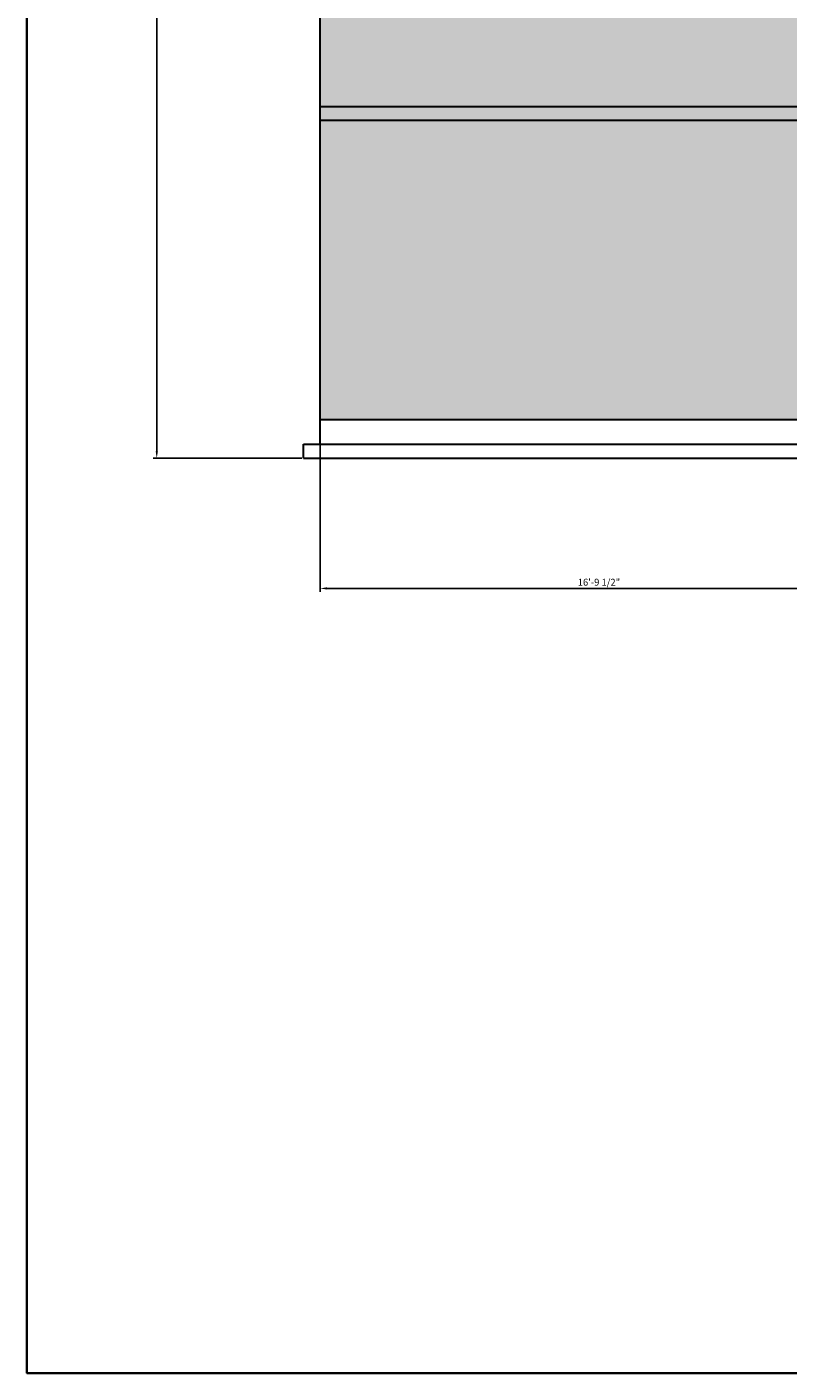
# Model space of a CAD drawing. Units: inches. Extents: x 2391 to 16591, y 7259 to 10239.
# Tile 1 of 27: x 2391 to 2666, y 7259 to 7745. Entities that reach past the tile are written whole.
import ezdxf

# ---------------------------------------------------------------- set-up
doc = ezdxf.new("R2010")
doc.units = ezdxf.units.IN
for name, color, linetype, lineweight in [('A-ANNO-DIMS', 4, 'Continuous', 18), ('A-ANNO-TTLB', 7, 'Continuous', 35), ('A-ELEV', 7, 'Continuous', 30), ('A-ELEV-PATT', 8, 'Continuous', 13), ('A-ELEV-SURF-PATT', 253, 'Continuous', 13)]:
    doc.layers.add(name, color=color, linetype=linetype, lineweight=lineweight)
doc.styles.get("Standard").update_dxf_attribs({"font": 'arial.ttf'})
doc.dimstyles.new('ISO-25', dxfattribs={"dimtxt": 2.5, "dimasz": 2.5, "dimexe": 1.25, "dimexo": 0.625, "dimtad": 1, "dimdec": 0, "dimlunit": 3, "dimtxsty": 'Standard', "dimcen": 2.5, "dimadec": 0, "dimazin": 0, "dimtfac": 1, "dimtdec": 0, "dimtmove": 0, "dimatfit": 3, "dimfxl": 1, "dimarcsym": 0})

# ---------------------------------------------------------------- blocks, each defined once
blk = doc.blocks.new('*D79')
at = {"layer": 'A-ANNO-DIMS', "color": 0, "lineweight": -2, "transparency": 16777216}
for p, q in [((2707.14, 8351.94), (2436.96, 8351.94)), ((2438.21, 7591.44), (2438.21, 8349.44)), ((2490.64, 7588.94), (2436.96, 7588.94))]:
    blk.add_line(p, q, dxfattribs=at)
at = {"layer": 'A-ANNO-DIMS', "color": 0, "transparency": 16777216}
for points in [[(2437.8, 8349.44), (2438.63, 8349.44), (2438.21, 8351.94)], [(2437.8, 7591.44), (2438.63, 7591.44), (2438.21, 7588.94)]]:
    blk.add_solid(points, dxfattribs=at)
at = {"layer": 'Defpoints', "color": 0, "transparency": 16777216}
for p in [(2438.21, 8351.94), (2707.76, 8351.94), (2491.26, 7588.94)]:
    blk.add_point(p, dxfattribs=at)
at = {"layer": 'A-ANNO-DIMS', "color": 0, "transparency": 16777216, "insert": (2436.31, 7970.44), "char_height": 2.5, "attachment_point": 5, "rotation": 90}
blk.add_mtext('63\'-7"', dxfattribs=at)
blk = doc.blocks.new('*D80')
at = {"layer": 'A-ANNO-DIMS', "color": 0, "lineweight": -2, "transparency": 16777216}
for p, q in [((2698.76, 7764.31), (2698.76, 7540.64)), ((2497.26, 7758.31), (2497.26, 7540.64)), ((2499.76, 7541.89), (2696.26, 7541.89))]:
    blk.add_line(p, q, dxfattribs=at)
at = {"layer": 'A-ANNO-DIMS', "color": 0, "transparency": 16777216}
for points in [[(2499.76, 7542.3), (2499.76, 7541.47), (2497.26, 7541.89)], [(2696.26, 7542.3), (2696.26, 7541.47), (2698.76, 7541.89)]]:
    blk.add_solid(points, dxfattribs=at)
at = {"layer": 'Defpoints', "color": 0, "transparency": 16777216}
for p in [(2698.76, 7764.94), (2497.26, 7758.94), (2698.76, 7541.89)]:
    blk.add_point(p, dxfattribs=at)
at = {"layer": 'A-ANNO-DIMS', "color": 0, "transparency": 16777216, "insert": (2598.01, 7543.8), "char_height": 2.5, "attachment_point": 5}
blk.add_mtext('16\'-9 1/2"', dxfattribs=at)

msp = doc.modelspace()

# ---------------------------------------------------------------- hatches: boundary and pattern name
at = {"layer": 'A-ELEV-PATT'}
h = msp.add_hatch(dxfattribs=at)
h.set_pattern_fill('GRAVEL', color=256)
h.paths.add_polyline_path([(2690.26, 7602.94), (2690.26, 7710.94), (2497.26, 7710.94), (2497.26, 7602.94)])
h.paths.add_polyline_path([(2929.26, 7710.94), (2857.26, 7710.94), (2857.26, 7602.94), (2929.26, 7602.94)])
at = {"layer": 'A-ELEV-SURF-PATT'}
h = msp.add_hatch(color=256, dxfattribs=at)
h.dxf.hatch_style = 1
h.paths.add_polyline_path([(2929.26, 7758.94), (2497.26, 7758.94), (2497.26, 7715.94), (2690.26, 7715.94), (2690.26, 7724.94), (2685.26, 7724.94), (2685.26, 7729.94), (2704.26, 7729.94), (2704.26, 7724.94), (2699.26, 7724.94), (2699.26, 7695.78), (2701.76, 7695.78), (2701.76, 7697.78), (2704.26, 7697.78), (2704.26, 7722.94), (2773.26, 7722.94), (2773.26, 7607.94), (2704.26, 7607.94), (2704.26, 7602.94), (2843.26, 7602.94), (2843.26, 7607.94), (2774.26, 7607.94), (2774.26, 7722.94), (2843.26, 7722.94), (2843.26, 7697.78), (2845.76, 7697.78), (2845.76, 7695.78), (2848.26, 7695.78), (2848.26, 7724.94), (2843.26, 7724.94), (2843.26, 7729.94), (2862.26, 7729.94), (2862.26, 7724.94), (2857.26, 7724.94), (2857.26, 7715.94), (2929.26, 7715.94)])
h.paths.add_polyline_path([(2848.26, 7693.78), (2845.76, 7693.78), (2845.76, 7691.78), (2843.26, 7691.78), (2843.26, 7637.65), (2845.76, 7637.65), (2845.76, 7635.65), (2848.26, 7635.65)], flags=17)
h.paths.add_polyline_path([(2848.26, 7633.65), (2845.76, 7633.65), (2845.76, 7631.65), (2843.26, 7631.65), (2843.26, 7602.94), (2848.26, 7602.94)], flags=17)
h.paths.add_polyline_path([(2704.26, 7631.65), (2701.76, 7631.65), (2701.76, 7633.65), (2699.26, 7633.65), (2699.26, 7602.94), (2704.26, 7602.94), (2704.26, 7607.94)], flags=17)
h.paths.add_polyline_path([(2704.26, 7691.78), (2701.76, 7691.78), (2701.76, 7693.78), (2699.26, 7693.78), (2699.26, 7635.65), (2701.76, 7635.65), (2701.76, 7637.65), (2704.26, 7637.65)], flags=17)
h = msp.add_hatch(color=256, dxfattribs=at)
h.dxf.hatch_style = 1
h.paths.add_polyline_path([(2690.26, 7715.94), (2497.26, 7715.94), (2497.26, 7710.94), (2690.26, 7710.94)])
h.paths.add_polyline_path([(2704.26, 7729.94), (2685.26, 7729.94), (2685.26, 7724.94), (2704.26, 7724.94)])
h.paths.add_polyline_path([(2862.26, 7729.94), (2843.26, 7729.94), (2843.26, 7724.94), (2862.26, 7724.94)])
h.paths.add_polyline_path([(2929.26, 7715.94), (2857.26, 7715.94), (2857.26, 7710.94), (2929.26, 7710.94)])

# ---------------------------------------------------------------- linework, layer by layer
at = {"layer": 'A-ANNO-TTLB'}
msp.add_lwpolyline([(2391.28, 10239.38), (4154.2, 10239.38), (4154.2, 7258.54), (2391.28, 7258.54)], close=True, dxfattribs=at)
at = {"layer": 'A-ELEV'}
for p, q in [((2497.26, 7593.94), (2497.26, 7758.94)), ((2497.26, 7715.94), (2690.26, 7715.94)), ((2497.26, 7710.94), (2690.26, 7710.94)), ((2497.26, 7602.94), (2929.26, 7602.94)), ((2491.26, 7593.94), (2935.26, 7593.94)), ((2491.26, 7588.94), (2491.26, 7593.94)), ((2491.26, 7588.94), (2935.26, 7588.94))]:
    msp.add_line(p, q, dxfattribs=at)

# ---------------------------------------------------------------- dimensions: what is measured, and where the dimension line sits
at = {"layer": 'A-ANNO-DIMS'}
dim = msp.add_linear_dim(base=(2438.21, 8351.94), p1=(2491.26, 7588.94), p2=(2707.76, 8351.94), angle=90, dimstyle='ISO-25', override={"dimdec": 1, "dimlfac": 1, "dimrnd": 0, "dimzin": 1, "dimdsep": 46, "dimlunit": 4, "dimfrac": 2}, dxfattribs=at)
dim.commit()
dim.dimension.update_dxf_attribs({"geometry": '*D79', "text_midpoint": (2436.31, 7970.44)})
dim = msp.add_linear_dim(base=(2698.76, 7541.89), p1=(2497.26, 7758.94), p2=(2698.76, 7764.94), dimstyle='ISO-25', override={"dimdec": 1, "dimlfac": 1, "dimrnd": 0, "dimzin": 1, "dimdsep": 46, "dimlunit": 4, "dimfrac": 2}, dxfattribs=at)
dim.commit()
dim.dimension.update_dxf_attribs({"geometry": '*D80', "text_midpoint": (2598.01, 7543.8)})

doc.saveas('drawing.dxf')
